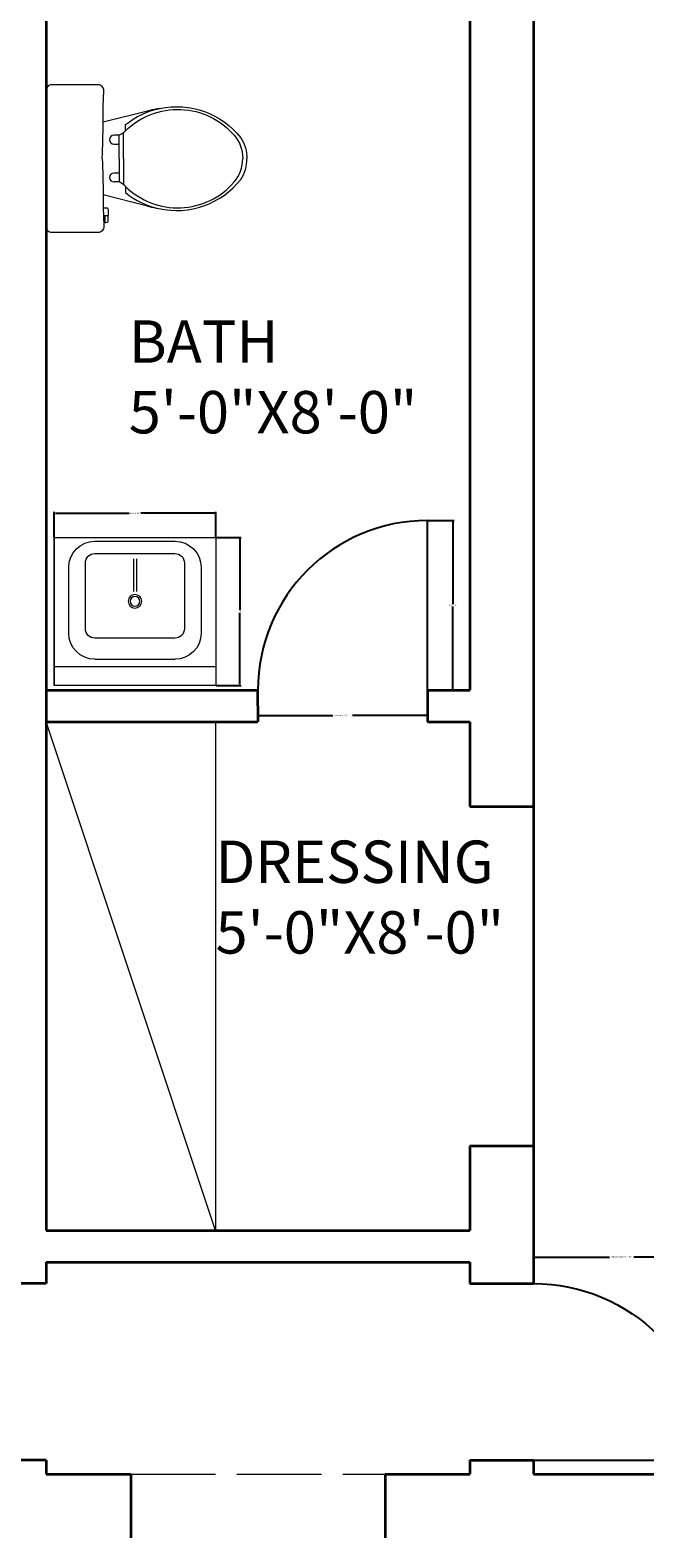
# Model space of a CAD drawing. Units: inches. Extents: x -10 to 502, y -868 to 56.
# Tile 12 of 14: x 211 to 298, y -264 to -50. Entities that reach past the tile are written whole.
import ezdxf

# ---------------------------------------------------------------- set-up
doc = ezdxf.new("R2010")
doc.units = ezdxf.units.IN
doc.header["$MEASUREMENT"] = 0
doc.linetypes.add('ACAD_ISO02W100', pattern=[15, 12, -3])
for name, color, linetype, lineweight in [('A-ANNO-DIMS', 2, 'Continuous', 18), ('A-AREA-IDEN', 7, 'Continuous', 18), ('A-DOOR', 4, 'Continuous', 25), ('A-FLOR-CASE', 8, 'Continuous', 18), ('A-FLOR-FIXT', 8, 'Continuous', 18), ('A-WALL', 7, 'Continuous', 35), ('A-WALL-OVHD', 7, 'ACAD_ISO02W100', 18), ('WC-Detail_dwgmodels.com', 251, 'Continuous', 13), ('WC-Outline_dwgmodels.com', 250, 'Continuous', 18)]:
    doc.layers.add(name, color=color, linetype=linetype, lineweight=lineweight)
doc.styles.get("Standard").update_dxf_attribs({"font": 'arial.ttf'})
doc.dimstyles.get("Standard").update_dxf_attribs({"dimtxt": 0.18, "dimasz": 0.18, "dimexe": 0.18, "dimexo": 0.0625, "dimgap": 0.09, "dimtad": 0, "dimtih": 1, "dimtoh": 1, "dimdec": 0, "dimzin": 0, "dimdsep": 46, "dimlunit": 3, "dimtxsty": 'Standard', "dimcen": 0.09, "dimadec": 0, "dimazin": 0, "dimtfac": 1, "dimtdec": 0, "dimtofl": 0, "dimtmove": 0, "dimatfit": 3, "dimfxl": 1, "dimtolj": 1, "dimtzin": 0, "dimarcsym": 0})

# ---------------------------------------------------------------- blocks, each defined once
blk = doc.blocks.new('М14 600х655')
for p, q in [((-655, 600), (-655, 0)), ((-655, 600), (-655, 0)), ((-655, 0), (-655, 600)), ((0, 600), (-655, 600)), ((0, 0), (0, 600)), ((0, 525), (-655, 525)), ((-165.1, 494.1), (-489.9, 494.1)), ((-595.8, 388.1), (-595.8, 121.3)), ((-528.4, 370.1), (-528.4, 103.3)), ((-165.4, 408.4), (-490.2, 408.4)), ((-127.2, 103.3), (-127.2, 370.1)), ((-59.2, 121.3), (-59.2, 388.1)), ((-333.5, 87.1), (-333.5, 219.6)), ((-321.5, 87.1), (-321.5, 219.6)), ((-490.2, 65.1), (-165.4, 65.1)), ((-655, 0), (-655, 0)), ((-655, 0), (-655, 0)), ((-655, 0), (0, 0)), ((-655, 0), (0, 0)), ((-489.9, 15.4), (-165.1, 15.4))]:
    blk.add_line(p, q)
for radius in [27.6, 19.3]:
    blk.add_circle((-327.5, 258.9), radius)
for centre, radius, start, end in [((-489.9, 388.1), 105.9, 90, 180), ((-165.1, 388.1), 105.9, 0, 90), ((-490.2, 370.1), 38.2, 90, 180), ((-165.4, 370.1), 38.2, 0, 90), ((-489.9, 121.3), 105.9, 180, 270), ((-490.2, 103.3), 38.2, 180, 270), ((-165.4, 103.3), 38.2, 270, 0), ((-165.1, 121.3), 105.9, 270, 0)]:
    blk.add_arc(centre, radius, start, end)
blk = doc.blocks.new('DOOR-SWING-24IN')
blk.add_line((24, 0), (24, 24))
blk.add_arc((24, 0), 24, 90, 180)
blk = doc.blocks.new('DOOR-SWING-25IN')
blk.add_line((25, 0), (0, 0))
blk.add_arc((25, 0), 25, 90, 180)
blk = doc.blocks.new('*D23')
at = {"layer": 'A-ANNO-DIMS', "color": 0, "lineweight": -2, "transparency": 16777216}
for p, q in [((243.45, -143.92), (243.45, -147.63)), ((267.45, -143.92), (267.45, -147.63)), ((243.63, -147.45), (254.06, -147.45)), ((267.27, -147.45), (256.85, -147.45))]:
    blk.add_line(p, q, dxfattribs=at)
at = {"layer": 'A-ANNO-DIMS', "color": 0, "transparency": 16777216}
for points in [[(243.63, -147.42), (243.63, -147.48), (243.45, -147.45)], [(267.27, -147.42), (267.27, -147.48), (267.45, -147.45)]]:
    blk.add_solid(points, dxfattribs=at)
at = {"layer": 'Defpoints', "color": 0, "transparency": 16777216}
for p in [(243.45, -143.85), (267.45, -143.85), (267.45, -147.45)]:
    blk.add_point(p, dxfattribs=at)
at = {"layer": 'A-ANNO-DIMS', "color": 0, "transparency": 16777216, "insert": (255.45, -147.45), "char_height": 0.18, "attachment_point": 5}
blk.add_mtext('\\A1;DOOR LEAF 2\'-0" TYP.', dxfattribs=at)
blk = doc.blocks.new('*D24')
at = {"layer": 'A-ANNO-DIMS', "color": 0, "lineweight": -2, "transparency": 16777216}
for p, q in [((267.51, -119.85), (271.23, -119.85)), ((271.05, -120.03), (271.05, -131.67)), ((271.05, -143.67), (271.05, -132.03)), ((267.51, -143.85), (271.23, -143.85))]:
    blk.add_line(p, q, dxfattribs=at)
at = {"layer": 'A-ANNO-DIMS', "color": 0, "transparency": 16777216}
for points in [[(271.02, -120.03), (271.08, -120.03), (271.05, -119.85)], [(271.02, -143.67), (271.08, -143.67), (271.05, -143.85)]]:
    blk.add_solid(points, dxfattribs=at)
at = {"layer": 'Defpoints', "color": 0, "transparency": 16777216}
for p in [(267.45, -119.85), (271.05, -119.85), (267.45, -143.85)]:
    blk.add_point(p, dxfattribs=at)
at = {"layer": 'A-ANNO-DIMS', "color": 0, "transparency": 16777216, "insert": (271.05, -131.85), "char_height": 0.18, "attachment_point": 5}
blk.add_mtext('\\A1;2\'-0" TYP.', dxfattribs=at)
blk = doc.blocks.new('*D25')
at = {"layer": 'A-ANNO-DIMS', "color": 0, "lineweight": -2, "transparency": 16777216}
for p, q in [((282.45, -227.79), (282.45, -223.92)), ((307.45, -227.79), (307.45, -223.92)), ((282.63, -224.1), (293.22, -224.1)), ((307.27, -224.1), (296.68, -224.1))]:
    blk.add_line(p, q, dxfattribs=at)
at = {"layer": 'A-ANNO-DIMS', "color": 0, "transparency": 16777216}
for points in [[(282.63, -224.07), (282.63, -224.13), (282.45, -224.1)], [(307.27, -224.07), (307.27, -224.13), (307.45, -224.1)]]:
    blk.add_solid(points, dxfattribs=at)
at = {"layer": 'Defpoints', "color": 0, "transparency": 16777216}
for p in [(282.45, -224.1), (282.45, -227.85), (307.45, -227.85)]:
    blk.add_point(p, dxfattribs=at)
at = {"layer": 'A-ANNO-DIMS', "color": 0, "transparency": 16777216, "insert": (294.95, -224.1), "char_height": 0.18, "attachment_point": 5}
blk.add_mtext('\\A1;BEDROOM DOOR 2\'-1" TYP.', dxfattribs=at)
blk = doc.blocks.new('*D31')
at = {"layer": 'A-ANNO-DIMS', "color": 0, "lineweight": -2, "transparency": 16777216}
for p, q in [((214.61, -122.18), (214.61, -118.63)), ((214.79, -118.81), (225.24, -118.81)), ((237.3, -118.81), (226.85, -118.81)), ((237.48, -122.18), (237.48, -118.63))]:
    blk.add_line(p, q, dxfattribs=at)
at = {"layer": 'A-ANNO-DIMS', "color": 0, "transparency": 16777216}
for points in [[(214.79, -118.78), (214.79, -118.84), (214.61, -118.81)], [(237.3, -118.78), (237.3, -118.84), (237.48, -118.81)]]:
    blk.add_solid(points, dxfattribs=at)
at = {"layer": 'Defpoints', "color": 0, "transparency": 16777216}
for p in [(237.48, -118.81), (214.61, -122.24), (237.48, -122.24)]:
    blk.add_point(p, dxfattribs=at)
at = {"layer": 'A-ANNO-DIMS', "color": 0, "transparency": 16777216, "insert": (226.04, -118.81), "char_height": 0.18, "attachment_point": 5}
blk.add_mtext('\\A1;BASIN 1\'-11"', dxfattribs=at)
blk = doc.blocks.new('*D32')
at = {"layer": 'A-ANNO-DIMS', "color": 0, "lineweight": -2, "transparency": 16777216}
for p, q in [((237.54, -122.24), (241.09, -122.24)), ((240.91, -122.42), (240.91, -132.53)), ((240.91, -143.01), (240.91, -132.9)), ((237.54, -143.19), (241.09, -143.19))]:
    blk.add_line(p, q, dxfattribs=at)
at = {"layer": 'A-ANNO-DIMS', "color": 0, "transparency": 16777216}
for points in [[(240.88, -122.42), (240.94, -122.42), (240.91, -122.24)], [(240.88, -143.01), (240.94, -143.01), (240.91, -143.19)]]:
    blk.add_solid(points, dxfattribs=at)
at = {"layer": 'Defpoints', "color": 0, "transparency": 16777216}
for p in [(237.48, -122.24), (237.48, -143.19), (240.91, -143.19)]:
    blk.add_point(p, dxfattribs=at)
at = {"layer": 'A-ANNO-DIMS', "color": 0, "transparency": 16777216, "insert": (240.91, -132.72), "char_height": 0.18, "attachment_point": 5}
blk.add_mtext('\\A1;1\'-9"', dxfattribs=at)

msp = doc.modelspace()

# ---------------------------------------------------------------- linework, layer by layer
at = {"layer": 'A-FLOR-CASE'}
for p, q in [((237.45, -220.35), (213.45, -148.35)), ((237.45, -148.35), (237.45, -220.35))]:
    msp.add_line(p, q, dxfattribs=at)
at = {"layer": 'A-WALL'}
for p, q in [((213.45, -47.85), (213.45, -143.85)), ((273.45, -47.85), (273.45, -143.85)), ((282.45, -47.85), (282.45, -227.85)), ((213.45, -143.85), (243.45, -143.85)), ((213.45, -143.85), (213.45, -148.35)), ((243.45, -146.1), (243.45, -143.85)), ((267.45, -143.85), (267.45, -148.35)), ((267.45, -143.85), (273.45, -143.85)), ((243.45, -146.1), (243.45, -148.35)), ((213.45, -148.35), (243.45, -148.35)), ((213.45, -148.35), (213.45, -220.35)), ((267.45, -148.35), (273.45, -148.35)), ((273.45, -148.35), (273.45, -160.35)), ((273.45, -160.35), (282.45, -160.35)), ((273.45, -208.35), (282.45, -208.35)), ((273.45, -208.35), (273.45, -220.35)), ((213.45, -220.35), (273.45, -220.35)), ((213.45, -224.85), (273.45, -224.85)), ((213.45, -224.85), (213.45, -227.85)), ((273.45, -224.85), (273.45, -227.85)), ((213.45, -227.85), (204.45, -227.85)), ((273.45, -227.85), (282.45, -227.85)), ((213.45, -252.85), (204.45, -252.85)), ((213.45, -252.85), (213.45, -254.85)), ((273.45, -252.85), (282.45, -252.85)), ((273.45, -252.85), (273.45, -254.85)), ((282.45, -252.85), (282.45, -254.85)), ((213.45, -254.85), (225.45, -254.85)), ((225.45, -254.85), (225.45, -263.85)), ((261.45, -254.85), (261.45, -263.85)), ((261.45, -254.85), (273.45, -254.85)), ((282.45, -254.85), (448.95, -254.85))]:
    msp.add_line(p, q, dxfattribs=at)
at = {"layer": 'A-WALL-OVHD'}
msp.add_line((225.45, -254.85), (261.45, -254.85), dxfattribs=at)
at = {"layer": 'WC-Detail_dwgmodels.com'}
for p, q in [((223.79, -65.31), (223.08, -65.31)), ((224.44, -64.96), (223.79, -65.31)), ((223.79, -66.58), (223.79, -65.31)), ((223.08, -66.58), (223.79, -66.58)), ((223.79, -68.62), (223.79, -66.58)), ((223.79, -68.62), (223.79, -70.65)), ((223.08, -70.65), (223.79, -70.65)), ((223.79, -71.92), (223.08, -71.92)), ((223.79, -70.65), (223.79, -71.92)), ((224.44, -72.28), (223.79, -71.92))]:
    msp.add_line(p, q, dxfattribs=at)
for points in [[(224.7, -63.8, -0.117999), (229.57, -61.51, -0.16845)], [(224.7, -64.68, -0.434217), (240.09, -65.31, -0.182634), (241.3, -68.62, -2.693815)], [(224.7, -64.68), (224.7, -63.8, -0.416606)], [(224.44, -64.96, -0.008985), (224.7, -64.68, -0.182634)], [(224.44, -68.62), (224.44, -64.96, -0.444938)], [(224.44, -68.62), (224.44, -72.28, 0.008985)], [(224.7, -72.55, 0.434217), (240.09, -71.92, 0.182634), (241.3, -68.62, 2.693815)], [(224.44, -72.28, 0.008985), (224.7, -72.55, 0.182634)], [(224.7, -72.55), (224.7, -73.43, 0.416606)], [(224.7, -73.43, 0.114632), (229.42, -75.69, 0.16845)]]:
    msp.add_lwpolyline(points, format="xyb", dxfattribs=at)
for centre in [(223.08, -65.94), (223.08, -71.29)]:
    msp.add_arc(centre, 0.635, 90, 270, dxfattribs=at)
at = {"layer": 'WC-Outline_dwgmodels.com'}
for points in [[(221.54, -63.48, 0.00511), (221.53, -61.19), (221.63, -59.01, 0.426005), (220.81, -58.15), (214.27, -58.15, 0.414214), (213.45, -58.97), (213.45, -68.61)], [(229.57, -61.51, 0.0272), (228.03, -61.83, 0.005151), (227.82, -61.89, 0.103607)], [(229.57, -61.51, -0.284616), (241.01, -65.66, -0.171216), (241.86, -68.62, -2.912347)], [(221.4, -68.6, 0.010344), (221.54, -63.48)], [(221.57, -76.69), (221.63, -78.22, -0.426005), (220.81, -79.07), (214.27, -79.07, -0.414214), (213.45, -78.25), (213.45, -68.61)], [(221.4, -68.62, -0.010344), (221.54, -73.74)], [(229.42, -75.69, 0.288211), (241.01, -71.57, 0.171216), (241.86, -68.62, 2.912232)], [(221.54, -73.74, -0.006773), (221.53, -75.47), (221.53, -75.61, -0.55454)], [(221.53, -75.61), (221.57, -76.69, -0.319616)], [(222.18, -76.69), (222.2, -76.69, 0.414214), (222.29, -76.6), (222.29, -75.87, 0.414214), (222.03, -75.61), (221.53, -75.61)], [(222.18, -76.69), (222.18, -77.55, -0.3351), (222.11, -77.64), (221.9, -77.7, -0.498015), (221.83, -77.64), (221.83, -76.69)], [(227.82, -75.33, 0.005151), (228.03, -75.39, 0.024565), (229.42, -75.69, 0.065413)]]:
    msp.add_lwpolyline(points, format="xyb", dxfattribs=at)
for points in [[(227.82, -61.89), (221.54, -63.48)], [(227.82, -75.33), (221.54, -73.74)], [(221.57, -76.69), (221.83, -76.69)], [(221.83, -76.69), (222.18, -76.69)]]:
    msp.add_lwpolyline(points, dxfattribs=at)

# ---------------------------------------------------------------- block references
at = {"layer": 'A-DOOR'}
msp.add_blockref('DOOR-SWING-24IN', (243.45, -143.85), dxfattribs=at)
at = {"layer": 'A-DOOR', "extrusion": (0, 0, -1), "zscale": -1}
msp.add_blockref('DOOR-SWING-25IN', (-307.45, -252.85), dxfattribs=at)
at = {"layer": 'A-FLOR-FIXT', "xscale": -0.03492429091277, "yscale": 0.03492429091277, "zscale": 0.03492429091277, "rotation": 180}
msp.add_blockref('М14 600х655', (237.48, -122.24), dxfattribs=at)

# ---------------------------------------------------------------- texts
at = {"layer": 'A-AREA-IDEN', "char_height": 6, "attachment_point": 1}
for s, insert in [('BATH\\P5\'-0"X8\'-0"', (225.16, -91.51)), ('DRESSING\\P5\'-0"X8\'-0"', (237.45, -165.15))]:
    msp.add_mtext(s, dxfattribs=dict(at, insert=insert))

# ---------------------------------------------------------------- dimensions: what is measured, and where the dimension line sits
at = {"layer": 'A-ANNO-DIMS'}
for base, p1, p2, text, picture, middle in [((237.48, -118.81), (214.61, -122.24), (237.48, -122.24), 'BASIN <>', '*D31', (226.04, -118.81)), ((267.45, -147.45), (243.45, -143.85), (267.45, -143.85), 'DOOR LEAF <> TYP.', '*D23', (255.45, -147.45))]:
    dim = msp.add_linear_dim(base=base, p1=p1, p2=p2, text=text, dimstyle='Standard', override={"dimdec": 1, "dimlfac": 1, "dimrnd": 0, "dimzin": 1, "dimdsep": 46, "dimlunit": 4, "dimfrac": 2}, dxfattribs=at)
    dim.commit()
    dim.dimension.update_dxf_attribs({"geometry": picture, "text_midpoint": middle})
for base, p1, p2, angle, text, picture, middle in [((271.05, -119.85), (267.45, -143.85), (267.45, -119.85), 90, '<> TYP.', '*D24', (271.05, -131.85)), ((282.45, -224.1), (307.45, -227.85), (282.45, -227.85), 180, 'BEDROOM DOOR <> TYP.', '*D25', (294.95, -224.1))]:
    dim = msp.add_linear_dim(base=base, p1=p1, p2=p2, angle=angle, text=text, dimstyle='Standard', override={"dimdec": 1, "dimlfac": 1, "dimrnd": 0, "dimzin": 1, "dimdsep": 46, "dimlunit": 4, "dimfrac": 2}, dxfattribs=at)
    dim.commit()
    dim.dimension.update_dxf_attribs({"geometry": picture, "text_midpoint": middle})
dim = msp.add_linear_dim(base=(240.9127, -143.193), p1=(237.4814, -122.2385), p2=(237.4814, -143.193), angle=270, dimstyle='Standard', override={"dimdec": 1, "dimlfac": 1, "dimrnd": 0, "dimzin": 1, "dimdsep": 46, "dimlunit": 4, "dimfrac": 2}, dxfattribs=at)
dim.commit()
dim.dimension.update_dxf_attribs({"geometry": '*D32', "text_midpoint": (240.9127, -132.7158)})

doc.saveas('drawing.dxf')
